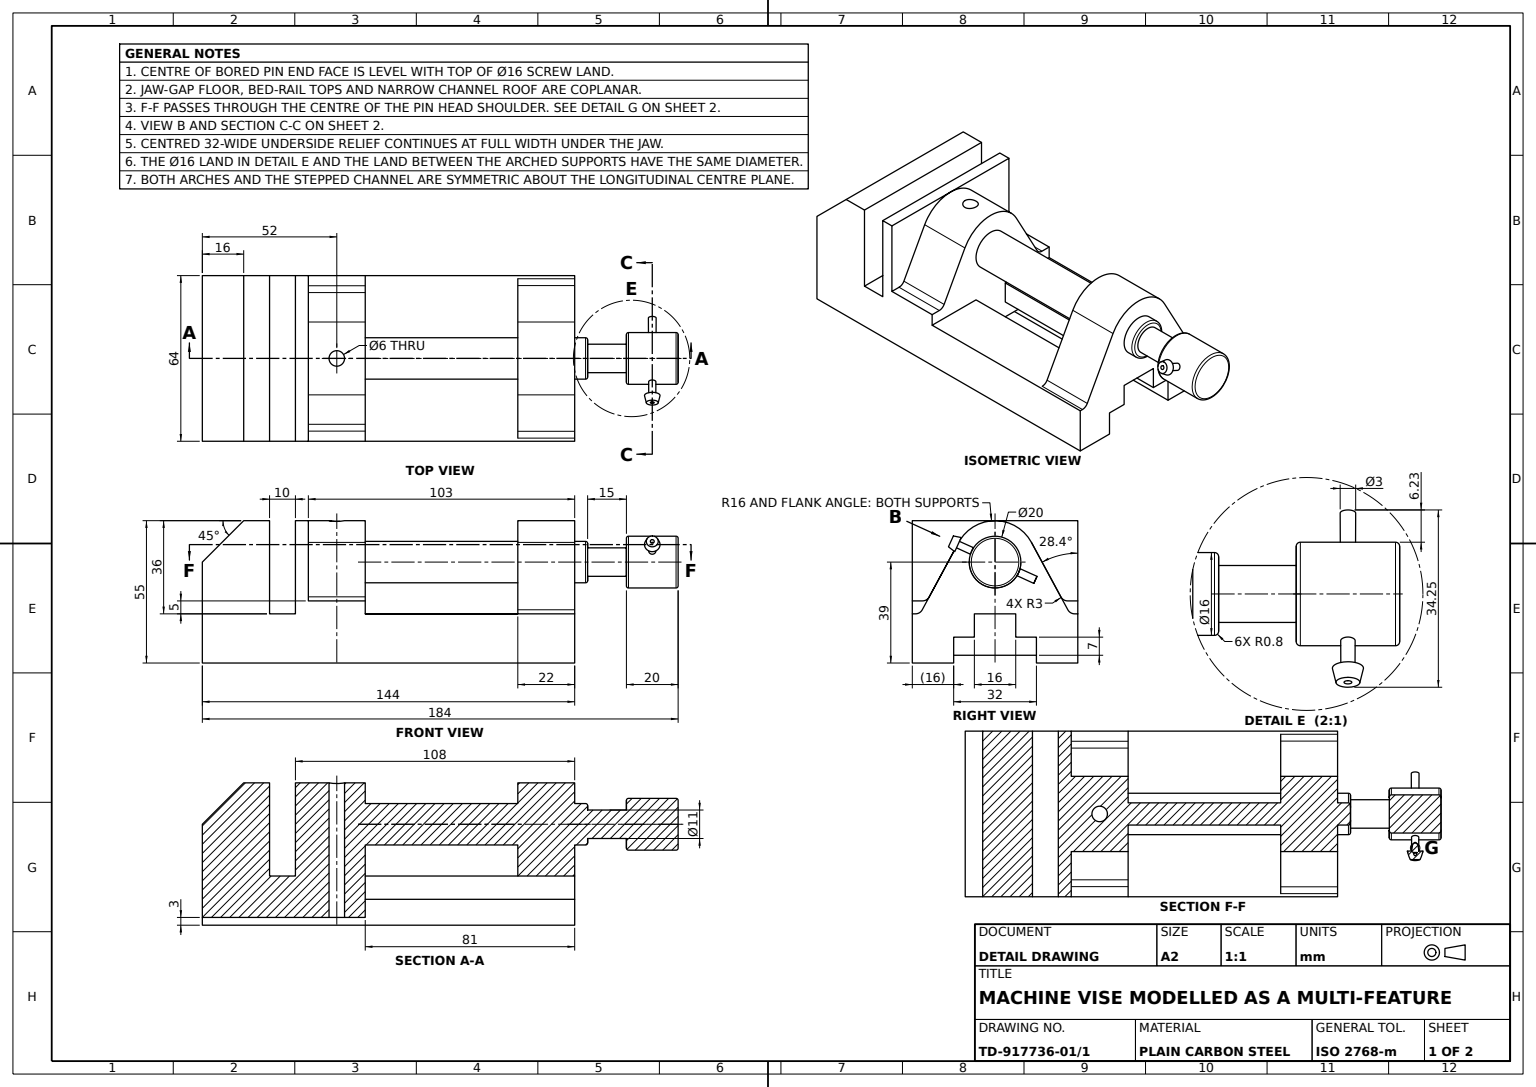
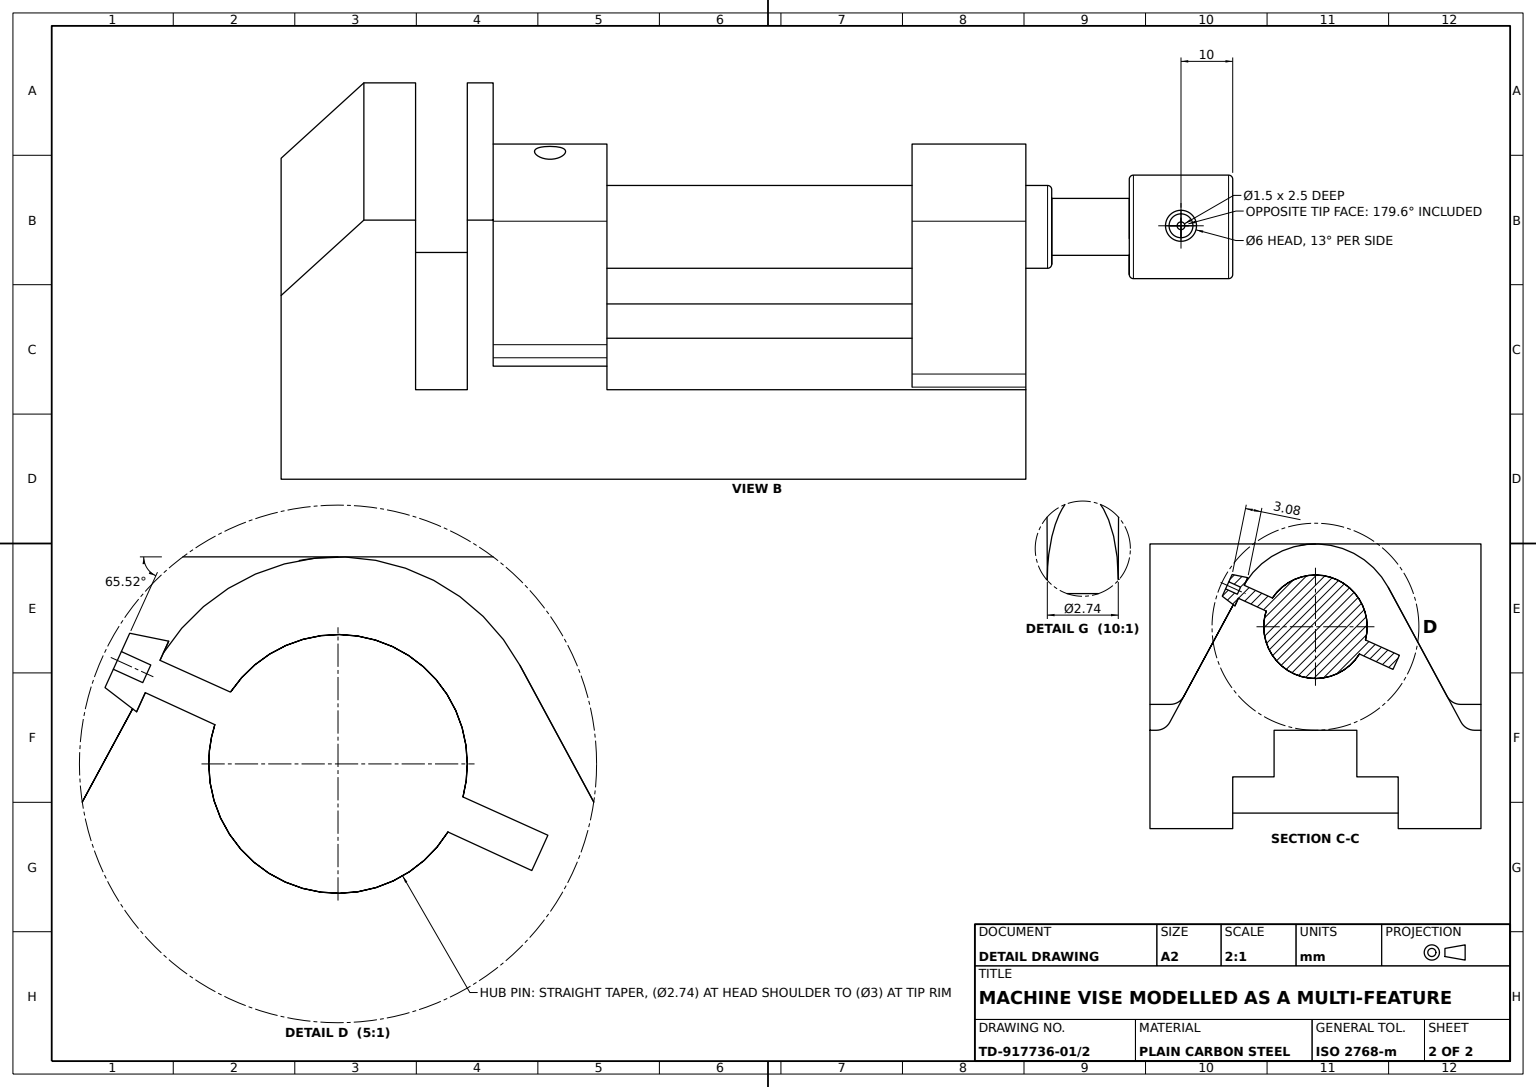
SolidWorks part; units mm, degrees
material "Plain Carbon Steel"
ref_plane "Front Plane" through (0, 0, 0) normal (0, 0, 1) x (1, 0, 0)
ref_plane "Top Plane" through (0, 0, 0) normal (0, 1, 0) x (1, 0, 0)
ref_plane "Right Plane" through (0, 0, 0) normal (1, 0, 0) x (0, 0, -1)
sketch "Vise Body Profile" plane through (0, 0, 0) normal (0, 0, 1) x (1, 0, 0)
  line L0 (0, 0) -> (0, 36)
  line L1 (0, 36) -> (16, 52)
  line L2 (16, 52) -> (26, 52)
  line L3 (26, 52) -> (26, 16)
  line L4 (26, 16) -> (122, 16)
  line L5 (122, 16) -> (122, 52)
  line L6 (122, 52) -> (144, 52)
  line L7 (144, 52) -> (144, 0)
  line L8 (144, 0) -> (0, 0)
  dimension "D1" = 16
  dimension "D2" = 16
  dimension "D3" = 16
  dimension "D4" = 10
  dimension "D5" = 36
  dimension "D6" = 22
  dimension "D7" = 144
extrude "Vise Body" add sketch "Vise Body Profile" along normal blind 64
sketch "Guide Channel Profile" plane through (144, 0, 0) normal (1, 0, 0) x (0, 0, -1)
  line L0 (-64, 0) -> (-48, 0)
  line L1 (-64, 0) -> (0, 0) construction
  line L2 (-48, 0) -> (-48, 7)
  line L3 (-48, 7) -> (-40, 7)
  line L4 (-40, 7) -> (-40, 16)
  line L5 (-40, 16) -> (-24, 16)
  line L6 (-24, 16) -> (-24, 7)
  line L7 (-24, 7) -> (-16, 7)
  line L8 (-16, 7) -> (-16, 0)
  line L9 (-16, 0) -> (0, 0)
  line L10 (-64, 0) -> (-64, 16)
  line L11 (-64, 16) -> (-61, 16)
  line L12 (-61, 16) -> (-46.075, 43.6088)
  line L13 (-17.925, 43.6088) -> (-3, 16)
  line L14 (-3, 16) -> (0, 16)
  line L15 (0, 16) -> (0, 0)
  arc A0 (-46.075, 43.6088) -> (-17.925, 43.6088) centre (-32, 36) cw
  point P5 (-32, 0)
  point P15 (-32, 16)
  dimension "D8" = 16
  dimension "D1" = 16
  dimension "D2" = 7
  dimension "D3" = 32
  dimension "D4" = 16
  dimension "D5" = 16
  dimension "D6" = 7
  dimension "D7" = 36
  dimension "D9" = 3
  dimension "D10" = 3
extrude "Guide Channel Cut" cut sketch "Guide Channel Profile" against normal blind 81 flip side to cut
ref_plane "Support Plate Plane" through (36, 0, 0) normal (1, 0, 0) x (0, 0, -1)
sketch "Support Plate Profile" plane through (36, 0, 0) normal (1, 0, 0) x (0, 0, -1)
  line L1 (-64, 0) -> (0, 0)
  line L2 (-64, 0) -> (-64, 52)
  line L3 (-64, 52) -> (0, 52)
  line L4 (0, 0) -> (0, 52)
extrude "Support Plate" add sketch "Support Plate Profile" along normal blind 5
ref_plane "Jaw Block Plane" through (41, 0, 0) normal (1, 0, 0) x (0, 0, -1)
sketch "Jaw Block Profile" plane through (41, 0, 0) normal (1, 0, 0) x (0, 0, -1)
  line L0 (-46.075, 43.6088) -> (-58.2971, 21)
  line L1 (-64, 16) -> (0, 16)
  line L2 (-17.925, 43.6088) -> (-5.7029, 21)
  line L3 (-3, 16) -> (-17.925, 43.6088) construction
  line L4 (-46.075, 43.6088) -> (-61, 16) construction
  line L5 (-58.2971, 21) -> (-64, 21)
  line L6 (-64, 52) -> (-64, 16) construction
  line L7 (-5.7029, 21) -> (0, 21)
  line L8 (0, 16) -> (0, 52) construction
  line L9 (-64, 21) -> (-64, 16)
  line L10 (0, 16) -> (0, 21)
  arc A0 (-17.925, 43.6088) -> (-46.075, 43.6088) centre (-32, 36) ccw
  dimension "D3" = 16
  dimension "D1" = 5
  dimension "D2" = 5
extrude "Jaw Block" add sketch "Jaw Block Profile" along normal blind 22
sketch "Lead Screw Profile Ø16" plane through (144, 0, 0) normal (1, 0, 0) x (0, 0, -1)
  circle A0 centre (-32, 36) radius 8
  dimension "D1" = 16
extrude "Lead Screw Shaft Ø16" add sketch "Lead Screw Profile Ø16" against normal blind 81 and the other way blind 5
sketch "Screw Neck Profile Ø11" plane through (149, 0, 0) normal (1, 0, 0) x (0, 0, -1)
  circle A0 centre (-32, 36) radius 5.5
  dimension "D1" = 11
extrude "Screw Neck Ø11" add sketch "Screw Neck Profile Ø11" along normal blind 15
sketch "Handle Hub Profile Ø20" plane through (164, 0, 0) normal (1, 0, 0) x (0, 0, -1)
  circle A0 centre (-32, 36) radius 10
  dimension "D1" = 20
extrude "Handle Hub Ø20" add sketch "Handle Hub Profile Ø20" along normal blind 20
fillet "Jaw Block Fillet R3" radius 3 1 edges at (52, 21, 58.2971)
fillet "Jaw Block Channel Fillet R3" radius 3 3 edges at (133, 16, 3) (52, 21, 5.7029) (133, 16, 61)
ref_plane "Collar Plane" through (174, 0, 0) normal (1, 0, 0) x (0, 0, -1)
sketch "Collar Revolve Profile" plane through (174, 0, 0) normal (1, 0, 0) x (0, 0, -1)
  line L0 (-45.7677, 44.004) -> (-15.7677, 30.4884)
  line L5 (0, 21) -> (0, 52) construction
  line L6 (-57.3711, 47.7785) -> (-13.3535, 27.7414) construction
  line L7 (-45.7677, 44.004) -> (-46.3361, 42.7553)
  line L8 (-46.3361, 42.7553) -> (-16.3839, 29.1208)
  line L9 (-16.3839, 29.1208) -> (-15.7677, 30.4884)
  line L10 (0, 52) -> (-32, 52) construction
  dimension "D1" = 1.5
  dimension "D2" = 21.5116
  dimension "D3" = 29.1208
  dimension "D4" = 15.7677
  dimension "D5" = 0.5684
  dimension "D6" = 29.9523
revolve "Collar Revolve" add sketch "Collar Revolve Profile" angle 360 about L6
sketch "Pin Boss Profile Ø6" plane through (0, 24.811, 54.5046) normal (0, 0.4143, 0.9101) x (1, 0, 0)
  circle A0 centre (174, 19.7161) radius 3
  dimension "D1" = 6
extrude "Pin Boss Ø6" add sketch "Pin Boss Profile Ø6" along normal blind 3 draft 13
sketch "Pin Hole Profile Ø1.5" plane through (0, 26.0539, 57.235) normal (0, 0.4143, 0.9101) x (1, 0, 0)
  circle A0 centre (174, 19.7161) radius 0.75
  dimension "D1" = 1.5
extrude "Pin Hole Ø1.5" cut sketch "Pin Hole Profile Ø1.5" against normal blind 2.5
sketch "Base Foot Profile" plane through (0, 0, 64) normal (0, 0, 1) x (1, 0, 0)
  line L0 (0, 0) -> (0, -3)
  line L1 (0, -3) -> (144, -3)
  line L2 (144, -3) -> (144, 0)
  line L3 (0, 0) -> (144, 0)
  dimension "D1" = 3
extrude "Base Foot" add sketch "Base Foot Profile" against normal blind 16
sketch "Foot Extension Profile" plane through (0, 0, 0) normal (0, 0, -1) x (-1, 0, 0)
  line L1 (0, -3) -> (-144, -3)
  line L2 (0, -3) -> (0, 0)
  line L3 (0, 0) -> (-144, 0)
  line L4 (-144, -3) -> (-144, 0)
extrude "Foot Extension" add sketch "Foot Extension Profile" against normal blind 16
sketch "Jaw Hole Profile Ø6" plane through (0, 0, 0) normal (0, -1, 0) x (1, 0, 0)
  line L0 (0, 48) -> (0, 16) construction
  circle A0 centre (52, 32) radius 3
  point P4 (0, 32)
  dimension "D2" = 6
  dimension "D1" = 52
extrude "Jaw Hole Ø6" cut sketch "Jaw Hole Profile Ø6" against normal blind 66
fillet "Handle Hub Fillet R0.8" radius 0.8 2 edges at (164, 36, 22) (184, 36, 22)
fillet "Lead Screw Fillet R0.8" radius 0.8 1 edges at (149, 36, 24)
